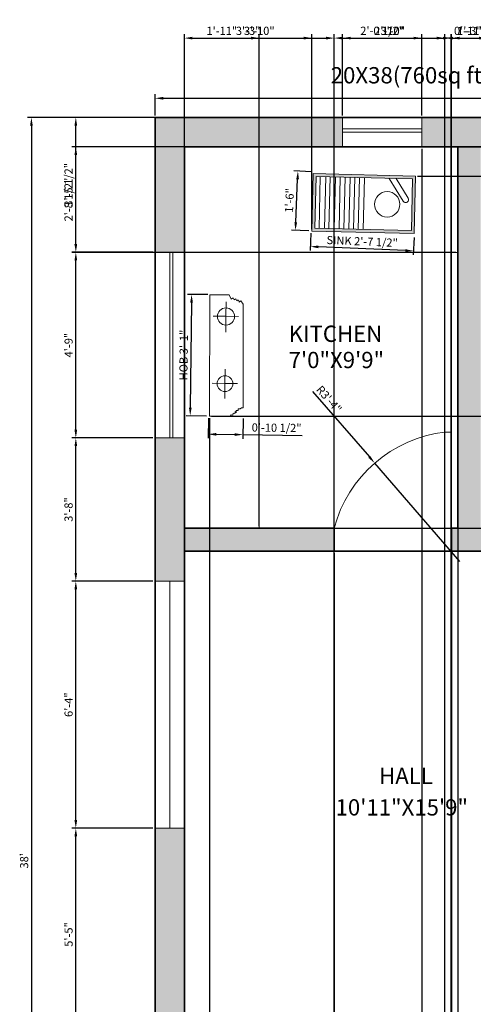
# Model space of a CAD drawing. Units: millimetres. Extents: x 2466 to 2817, y 2000 to 2512.
# Tile 3 of 4: x 2466 to 2605, y 2210 to 2512. Entities that reach past the tile are written whole.
import ezdxf

# ---------------------------------------------------------------- set-up
doc = ezdxf.new("R2010")
doc.units = ezdxf.units.MM
for name, color, linetype, lineweight in [('A-ANNO-DIMS', 2, 'Continuous', 13), ('A-ANNO-TEXT', 7, 'Continuous', 18), ('A-AREA-IDEN', 7, 'Continuous', 18), ('A-DOOR', 3, 'Continuous', 18), ('A-EQPM', 8, 'Continuous', 18), ('A-FLOR-FIXT', 9, 'Continuous', 18), ('A-GLAZ', 5, 'Continuous', 18), ('A-WALL', 7, 'Continuous', 35), ('A-WALL-PATT', 8, 'Continuous', 13)]:
    doc.layers.add(name, color=color, linetype=linetype, lineweight=lineweight)
doc.styles.get("Standard").update_dxf_attribs({"font": 'arial.ttf'})
doc.dimstyles.new('ISO-25', dxfattribs={"dimtxt": 2.5, "dimasz": 2.5, "dimexe": 1.25, "dimexo": 0.625, "dimtad": 1, "dimdec": 0, "dimlunit": 3, "dimtxsty": 'Standard', "dimcen": 2.5, "dimadec": 0, "dimazin": 0, "dimtfac": 1, "dimtdec": 0, "dimtmove": 0, "dimatfit": 3, "dimfxl": 1, "dimarcsym": 0})

# ---------------------------------------------------------------- blocks, each defined once
blk = doc.blocks.new('oven')
h = blk.add_hatch(color=256)
h.dxf.hatch_style = 1
h.paths.add_polyline_path([(0, 0), (-0.57, 31.4), (-18.19, 31.08), (-17.62, -0.32)])
h.paths.add_polyline_path([(-0.89, 0.86), (-16.76, 0.57), (-17.3, 30.22), (-1.42, 30.51)], flags=16)
h.paths.add_polyline_path([(-8.94, 4.45, -1), (-9.08, 12.23, -1)], flags=0)
for p, q in [((-1.42, 30.51), (-17.3, 30.22)), ((-1.4, 29.22), (-17.27, 28.94)), ((-1.37, 27.54), (-17.24, 27.26)), ((-1.35, 26.2), (-17.22, 25.91)), ((-1.32, 24.58), (-17.19, 24.29)), ((-1.29, 23.09), (-17.16, 22.8)), ((-1.26, 21.61), (-17.14, 21.33)), ((-1.24, 20.06), (-17.11, 19.77)), ((-1.21, 18.65), (-17.08, 18.36)), ((-1.19, 17.21), (-17.06, 16.92)), ((-1.16, 15.68), (-17.03, 15.4)), ((-1.02, 8.05), (-7.83, 3.46)), ((-8.14, 3.25), (-8.14, 3.25)), ((-0.98, 5.97), (-6.86, 2.02))]:
    blk.add_line(p, q)
for points in [[(-0.57, 31.4), (0, 0), (-17.62, -0.32), (-18.19, 31.08)], [(-1.42, 30.51), (-0.89, 0.86), (-16.76, 0.57), (-17.3, 30.22)]]:
    blk.add_lwpolyline(points, close=True)
blk.add_circle((-9.01, 8.34), 3.89)
blk.add_arc((-7.34, 2.74), 0.871, 123.9581, 303.9581)
blk = doc.blocks.new('gas stove')
for p, q in [((-59.95, 17.3), (-4.61, 17.86)), ((-4.61, 16.99), (-4.61, 17.86)), ((-4.03, 16.21), (-4.61, 16.99)), ((-4, 15.26), (-4.03, 16.21)), ((-0.18, 17.9), (-0.16, 17.9)), ((-53.37, 8.07), (-53.37, 14.75)), ((-53.37, 14.75), (-53.37, 1.35)), ((-17.48, 7.97), (-17.48, 14.65)), ((-17.48, 14.65), (-17.48, 1.25)), ((-3.18, 15.29), (-4, 15.26)), ((-3.15, 14.19), (-3.18, 15.29)), ((-1.96, 14.22), (-3.15, 14.19)), ((-2.6, 13.68), (-1.96, 14.22)), ((-1.52, 13.51), (-2.6, 13.68)), ((-1.66, 12.63), (-1.52, 13.51)), ((-0.57, 12.46), (-1.66, 12.63)), ((-0.73, 11.48), (-0.57, 12.46)), ((-0.11, 11.04), (-0.73, 11.48)), ((0, 0), (-0.11, 11.04)), ((0, 0), (-0.11, 11.04)), ((-64.71, -0.66), (-64.81, 9.74)), ((-64.71, -0.66), (-64.81, 9.74)), ((-53.37, 8.05), (-61.06, 8.07)), ((-53.37, 8.07), (-44.91, 8.07)), ((-53.37, 1.35), (-53.37, 8.05)), ((-17.48, 7.95), (-25.17, 7.97)), ((-17.48, 7.97), (-9.38, 7.97)), ((-17.48, 1.25), (-17.48, 7.95)), ((-64.71, -0.66), (0, 0))]:
    blk.add_line(p, q)
blk.add_lwpolyline([(-64.81, 9.74), (-62.59, 10.77), (-62.59, 10.77), (-63.19, 11.79), (-62.17, 12.38), (-62.65, 13.21), (-61.69, 13.77), (-62.14, 14.54), (-60.96, 15.22), (-61.23, 15.06), (-61.72, 15.9), (-59.95, 17.3)])
for centre, radius in [((-53.26, 8.13), 4.57), ((-17.38, 8.02), 4.19)]:
    blk.add_circle(centre, radius)
blk = doc.blocks.new('*D9')
at = {"layer": 'A-ANNO-DIMS', "color": 0, "lineweight": -2, "transparency": 16777216}
for p, q in [((2507.19, 2482.77), (2507.19, 2489.26)), ((2747.19, 2482.77), (2747.19, 2489.26)), ((2509.69, 2488.01), (2744.69, 2488.01))]:
    blk.add_line(p, q, dxfattribs=at)
at = {"layer": 'A-ANNO-DIMS', "color": 0, "transparency": 16777216}
for points in [[(2509.69, 2488.43), (2509.69, 2487.6), (2507.19, 2488.01)], [(2744.69, 2488.43), (2744.69, 2487.6), (2747.19, 2488.01)]]:
    blk.add_solid(points, dxfattribs=at)
at = {"layer": 'Defpoints', "color": 0, "transparency": 16777216}
for p in [(2747.19, 2488.01), (2507.19, 2482.15), (2747.19, 2482.15)]:
    blk.add_point(p, dxfattribs=at)
at = {"layer": 'A-ANNO-DIMS', "color": 0, "transparency": 16777216, "insert": (2627.19, 2489.92), "char_height": 2.5, "attachment_point": 5}
blk.add_mtext("20'", dxfattribs=at)
blk = doc.blocks.new('*D10')
at = {"layer": 'A-ANNO-DIMS', "color": 0, "lineweight": -2, "transparency": 16777216}
for p, q in [((2746.56, 2482.15), (2467.98, 2482.15)), ((2469.23, 2479.65), (2469.23, 2028.65)), ((2746.56, 2026.15), (2467.98, 2026.15))]:
    blk.add_line(p, q, dxfattribs=at)
at = {"layer": 'A-ANNO-DIMS', "color": 0, "transparency": 16777216}
for points in [[(2468.82, 2479.65), (2469.65, 2479.65), (2469.23, 2482.15)], [(2468.82, 2028.65), (2469.65, 2028.65), (2469.23, 2026.15)]]:
    blk.add_solid(points, dxfattribs=at)
at = {"layer": 'Defpoints', "color": 0, "transparency": 16777216}
for p in [(2747.19, 2482.15), (2469.23, 2026.15), (2747.19, 2026.15)]:
    blk.add_point(p, dxfattribs=at)
at = {"layer": 'A-ANNO-DIMS', "color": 0, "transparency": 16777216, "insert": (2467.33, 2254.15), "char_height": 2.5, "attachment_point": 5, "rotation": 90}
blk.add_mtext("38'", dxfattribs=at)
blk = doc.blocks.new('*D14')
at = {"layer": 'A-ANNO-DIMS', "color": 0, "lineweight": -2, "transparency": 16777216}
for p, q in [((2523.38, 2427.8), (2517.18, 2427.87)), ((2518.4, 2425.35), (2518.02, 2393.13)), ((2522.95, 2390.57), (2516.74, 2390.64))]:
    blk.add_line(p, q, dxfattribs=at)
at = {"layer": 'A-ANNO-DIMS', "color": 0, "transparency": 16777216}
for points in [[(2517.98, 2425.36), (2518.81, 2425.35), (2518.43, 2427.85)], [(2517.6, 2393.13), (2518.44, 2393.12), (2517.99, 2390.63)]]:
    blk.add_solid(points, dxfattribs=at)
at = {"layer": 'Defpoints', "color": 0, "transparency": 16777216}
for p in [(2524.01, 2427.79), (2517.99, 2390.63), (2523.58, 2390.56)]:
    blk.add_point(p, dxfattribs=at)
at = {"layer": 'A-ANNO-DIMS', "color": 0, "transparency": 16777216, "insert": (2516.29, 2409.26), "char_height": 2.5, "attachment_point": 5, "rotation": 89.3309}
blk.add_mtext('HOB 3\'-1"', dxfattribs=at)
blk = doc.blocks.new('*D15')
at = {"layer": 'A-ANNO-DIMS', "color": 0, "lineweight": -2, "transparency": 16777216}
for p, q in [((2523.57, 2389.94), (2523.5, 2383.73)), ((2534.23, 2389.81), (2534.16, 2383.6)), ((2526.01, 2384.95), (2531.67, 2384.88)), ((2534.17, 2384.85), (2552.33, 2384.64))]:
    blk.add_line(p, q, dxfattribs=at)
at = {"layer": 'A-ANNO-DIMS', "color": 0, "transparency": 16777216}
for points in [[(2526.01, 2385.37), (2526, 2384.53), (2523.51, 2384.98)], [(2531.68, 2385.3), (2531.67, 2384.47), (2534.17, 2384.85)]]:
    blk.add_solid(points, dxfattribs=at)
at = {"layer": 'Defpoints', "color": 0, "transparency": 16777216}
for p in [(2523.58, 2390.56), (2534.24, 2390.44), (2534.17, 2384.85)]:
    blk.add_point(p, dxfattribs=at)
at = {"layer": 'A-ANNO-DIMS', "color": 0, "transparency": 16777216, "insert": (2544.52, 2386.65), "char_height": 2.5, "attachment_point": 5, "rotation": 359.3309}
blk.add_mtext('0\'-10 1/2"', dxfattribs=at)
blk = doc.blocks.new('*D16')
at = {"layer": 'A-ANNO-DIMS', "color": 0, "lineweight": -2, "transparency": 16777216}
for p, q in [((2555.03, 2446.67), (2554.8, 2441.3)), ((2586.72, 2445.34), (2586.49, 2439.96)), ((2584.05, 2441.31), (2557.35, 2442.44))]:
    blk.add_line(p, q, dxfattribs=at)
at = {"layer": 'A-ANNO-DIMS', "color": 0, "transparency": 16777216}
for points in [[(2557.37, 2442.86), (2557.33, 2442.02), (2554.85, 2442.54)], [(2584.06, 2441.73), (2584.03, 2440.9), (2586.54, 2441.21)]]:
    blk.add_solid(points, dxfattribs=at)
at = {"layer": 'Defpoints', "color": 0, "transparency": 16777216}
for p in [(2555.05, 2447.3), (2586.74, 2445.96), (2554.85, 2442.54)]:
    blk.add_point(p, dxfattribs=at)
at = {"layer": 'A-ANNO-DIMS', "color": 0, "transparency": 16777216, "insert": (2570.78, 2443.79), "char_height": 2.5, "attachment_point": 5, "rotation": 357.5814}
blk.add_mtext('SINK 2\'-7 1/2"', dxfattribs=at)
blk = doc.blocks.new('*D17')
at = {"layer": 'A-ANNO-DIMS', "color": 0, "lineweight": -2, "transparency": 16777216}
for p, q in [((2555.2, 2465.5), (2549.82, 2465.72)), ((2550.41, 2450), (2550.96, 2463.17)), ((2554.43, 2447.32), (2549.05, 2447.55))]:
    blk.add_line(p, q, dxfattribs=at)
at = {"layer": 'A-ANNO-DIMS', "color": 0, "transparency": 16777216}
for points in [[(2550.55, 2463.19), (2551.38, 2463.15), (2551.07, 2465.67)], [(2549.99, 2450.01), (2550.82, 2449.98), (2550.3, 2447.5)]]:
    blk.add_solid(points, dxfattribs=at)
at = {"layer": 'Defpoints', "color": 0, "transparency": 16777216}
for p in [(2551.07, 2465.67), (2555.82, 2465.47), (2555.05, 2447.3)]:
    blk.add_point(p, dxfattribs=at)
at = {"layer": 'A-ANNO-DIMS', "color": 0, "transparency": 16777216, "insert": (2548.79, 2456.66), "char_height": 2.5, "attachment_point": 5, "rotation": 87.5814}
blk.add_mtext('1\'-6"', dxfattribs=at)
blk = doc.blocks.new('*D31')
at = {"layer": 'A-ANNO-DIMS', "color": 0, "lineweight": -2, "transparency": 16777216}
for p, q in [((2506.56, 2264.15), (2481.62, 2264.15)), ((2482.87, 2201.47), (2482.87, 2261.65)), ((2506.56, 2198.97), (2481.62, 2198.97))]:
    blk.add_line(p, q, dxfattribs=at)
at = {"layer": 'A-ANNO-DIMS', "color": 0, "transparency": 16777216}
for points in [[(2482.45, 2261.65), (2483.28, 2261.65), (2482.87, 2264.15)], [(2482.45, 2201.47), (2483.28, 2201.47), (2482.87, 2198.97)]]:
    blk.add_solid(points, dxfattribs=at)
at = {"layer": 'Defpoints', "color": 0, "transparency": 16777216}
for p in [(2482.87, 2264.15), (2507.19, 2264.15), (2507.19, 2198.97)]:
    blk.add_point(p, dxfattribs=at)
at = {"layer": 'A-ANNO-DIMS', "color": 0, "transparency": 16777216, "insert": (2480.97, 2231.56), "char_height": 2.5, "attachment_point": 5, "rotation": 90}
blk.add_mtext('5\'-5"', dxfattribs=at)
blk = doc.blocks.new('*D32')
at = {"layer": 'A-ANNO-DIMS', "color": 0, "lineweight": -2, "transparency": 16777216}
for p, q in [((2506.56, 2339.92), (2481.62, 2339.92)), ((2482.87, 2266.65), (2482.87, 2337.42)), ((2506.56, 2264.15), (2481.62, 2264.15))]:
    blk.add_line(p, q, dxfattribs=at)
at = {"layer": 'A-ANNO-DIMS', "color": 0, "transparency": 16777216}
for points in [[(2482.45, 2337.42), (2483.28, 2337.42), (2482.87, 2339.92)], [(2482.45, 2266.65), (2483.28, 2266.65), (2482.87, 2264.15)]]:
    blk.add_solid(points, dxfattribs=at)
at = {"layer": 'Defpoints', "color": 0, "transparency": 16777216}
for p in [(2482.87, 2339.92), (2507.19, 2339.92), (2507.19, 2264.15)]:
    blk.add_point(p, dxfattribs=at)
at = {"layer": 'A-ANNO-DIMS', "color": 0, "transparency": 16777216, "insert": (2480.97, 2302.03), "char_height": 2.5, "attachment_point": 5, "rotation": 90}
blk.add_mtext('6\'-4"', dxfattribs=at)
blk = doc.blocks.new('*D33')
at = {"layer": 'A-ANNO-DIMS', "color": 0, "lineweight": -2, "transparency": 16777216}
for p, q in [((2506.56, 2383.84), (2481.62, 2383.84)), ((2482.87, 2342.42), (2482.87, 2381.34)), ((2506.56, 2339.92), (2481.62, 2339.92))]:
    blk.add_line(p, q, dxfattribs=at)
at = {"layer": 'A-ANNO-DIMS', "color": 0, "transparency": 16777216}
for points in [[(2482.45, 2381.34), (2483.28, 2381.34), (2482.87, 2383.84)], [(2482.45, 2342.42), (2483.28, 2342.42), (2482.87, 2339.92)]]:
    blk.add_solid(points, dxfattribs=at)
at = {"layer": 'Defpoints', "color": 0, "transparency": 16777216}
for p in [(2482.87, 2383.84), (2507.19, 2383.84), (2507.19, 2339.92)]:
    blk.add_point(p, dxfattribs=at)
at = {"layer": 'A-ANNO-DIMS', "color": 0, "transparency": 16777216, "insert": (2480.96, 2361.88), "char_height": 2.5, "attachment_point": 5, "rotation": 90}
blk.add_mtext('3\'-8"', dxfattribs=at)
blk = doc.blocks.new('*D34')
at = {"layer": 'A-ANNO-DIMS', "color": 0, "lineweight": -2, "transparency": 16777216}
for p, q in [((2506.56, 2440.79), (2481.62, 2440.79)), ((2482.87, 2386.34), (2482.87, 2438.29)), ((2506.56, 2383.84), (2481.62, 2383.84))]:
    blk.add_line(p, q, dxfattribs=at)
at = {"layer": 'A-ANNO-DIMS', "color": 0, "transparency": 16777216}
for points in [[(2482.45, 2438.29), (2483.28, 2438.29), (2482.87, 2440.79)], [(2482.45, 2386.34), (2483.28, 2386.34), (2482.87, 2383.84)]]:
    blk.add_solid(points, dxfattribs=at)
at = {"layer": 'Defpoints', "color": 0, "transparency": 16777216}
for p in [(2482.87, 2440.79), (2507.19, 2440.79), (2507.19, 2383.84)]:
    blk.add_point(p, dxfattribs=at)
at = {"layer": 'A-ANNO-DIMS', "color": 0, "transparency": 16777216, "insert": (2480.97, 2412.31), "char_height": 2.5, "attachment_point": 5, "rotation": 90}
blk.add_mtext('4\'-9"', dxfattribs=at)
blk = doc.blocks.new('*D35')
at = {"layer": 'A-ANNO-DIMS', "color": 0, "lineweight": -2, "transparency": 16777216}
for p, q in [((2506.56, 2482.15), (2481.62, 2482.15)), ((2482.87, 2443.29), (2482.87, 2479.65)), ((2506.56, 2440.79), (2481.62, 2440.79))]:
    blk.add_line(p, q, dxfattribs=at)
at = {"layer": 'A-ANNO-DIMS', "color": 0, "transparency": 16777216}
for points in [[(2482.45, 2479.65), (2483.28, 2479.65), (2482.87, 2482.15)], [(2482.45, 2443.29), (2483.28, 2443.29), (2482.87, 2440.79)]]:
    blk.add_solid(points, dxfattribs=at)
at = {"layer": 'Defpoints', "color": 0, "transparency": 16777216}
for p in [(2482.87, 2482.15), (2507.19, 2482.15), (2507.19, 2440.79)]:
    blk.add_point(p, dxfattribs=at)
at = {"layer": 'A-ANNO-DIMS', "color": 0, "transparency": 16777216, "insert": (2480.95, 2461.47), "char_height": 2.5, "attachment_point": 5, "rotation": 90}
blk.add_mtext('3\'-5 1/2"', dxfattribs=at)
blk = doc.blocks.new('*D40')
at = {"layer": 'A-ANNO-DIMS', "color": 0, "lineweight": -2, "transparency": 16777216}
for p, q in [((2589.08, 2472.52), (2589.08, 2000.58)), ((2600.19, 2472.52), (2600.19, 2000.58)), ((2591.58, 2001.83), (2597.69, 2001.83))]:
    blk.add_line(p, q, dxfattribs=at)
at = {"layer": 'A-ANNO-DIMS', "color": 0, "transparency": 16777216}
for points in [[(2591.58, 2002.24), (2591.58, 2001.41), (2589.08, 2001.83)], [(2597.69, 2002.24), (2597.69, 2001.41), (2600.19, 2001.83)]]:
    blk.add_solid(points, dxfattribs=at)
at = {"layer": 'Defpoints', "color": 0, "transparency": 16777216}
for p in [(2589.08, 2473.15), (2600.19, 2473.15), (2600.19, 2001.83)]:
    blk.add_point(p, dxfattribs=at)
at = {"layer": 'A-ANNO-DIMS', "color": 0, "transparency": 16777216, "insert": (2594.63, 2003.73), "char_height": 2.5, "attachment_point": 5}
blk.add_mtext('0\'-11"', dxfattribs=at)
blk = doc.blocks.new('*D41')
at = {"layer": 'A-ANNO-DIMS', "color": 0, "lineweight": -2, "transparency": 16777216}
for p, q in [((2564.77, 2482.77), (2564.77, 2507.72)), ((2567.27, 2506.47), (2586.58, 2506.47)), ((2589.08, 2482.77), (2589.08, 2507.72))]:
    blk.add_line(p, q, dxfattribs=at)
at = {"layer": 'A-ANNO-DIMS', "color": 0, "transparency": 16777216}
for points in [[(2567.27, 2506.88), (2567.27, 2506.05), (2564.77, 2506.47)], [(2586.58, 2506.88), (2586.58, 2506.05), (2589.08, 2506.47)]]:
    blk.add_solid(points, dxfattribs=at)
at = {"layer": 'Defpoints', "color": 0, "transparency": 16777216}
for p in [(2589.08, 2506.47), (2564.77, 2482.15), (2589.08, 2482.15)]:
    blk.add_point(p, dxfattribs=at)
at = {"layer": 'A-ANNO-DIMS', "color": 0, "transparency": 16777216, "insert": (2576.93, 2508.39), "char_height": 2.5, "attachment_point": 5}
blk.add_mtext('2\'-0 1/2"', dxfattribs=at)
blk = doc.blocks.new('*D44')
at = {"layer": 'A-ANNO-DIMS', "color": 0, "lineweight": -2, "transparency": 16777216}
for p, q in [((2516.19, 2055.77), (2516.19, 2507.72)), ((2518.69, 2506.47), (2559.74, 2506.47)), ((2562.24, 2055.77), (2562.24, 2507.72))]:
    blk.add_line(p, q, dxfattribs=at)
at = {"layer": 'A-ANNO-DIMS', "color": 0, "transparency": 16777216}
for points in [[(2518.69, 2506.88), (2518.69, 2506.05), (2516.19, 2506.47)], [(2559.74, 2506.88), (2559.74, 2506.05), (2562.24, 2506.47)]]:
    blk.add_solid(points, dxfattribs=at)
at = {"layer": 'Defpoints', "color": 0, "transparency": 16777216}
for p in [(2562.24, 2506.47), (2516.19, 2055.15), (2562.24, 2055.15)]:
    blk.add_point(p, dxfattribs=at)
at = {"layer": 'A-ANNO-DIMS', "color": 0, "transparency": 16777216, "insert": (2539.21, 2508.37), "char_height": 2.5, "attachment_point": 5}
blk.add_mtext('3\'-10"', dxfattribs=at)
blk = doc.blocks.new('*D47')
at = {"layer": 'A-ANNO-DIMS', "color": 0, "lineweight": -2, "transparency": 16777216}
for p, q in [((2516.19, 2348.52), (2516.19, 2000.58)), ((2562.19, 2348.52), (2562.19, 2000.58)), ((2518.69, 2001.83), (2559.69, 2001.83))]:
    blk.add_line(p, q, dxfattribs=at)
at = {"layer": 'A-ANNO-DIMS', "color": 0, "transparency": 16777216}
for points in [[(2518.69, 2002.24), (2518.69, 2001.41), (2516.19, 2001.83)], [(2559.69, 2002.24), (2559.69, 2001.41), (2562.19, 2001.83)]]:
    blk.add_solid(points, dxfattribs=at)
at = {"layer": 'Defpoints', "color": 0, "transparency": 16777216}
for p in [(2516.19, 2349.15), (2562.19, 2349.15), (2562.19, 2001.83)]:
    blk.add_point(p, dxfattribs=at)
at = {"layer": 'A-ANNO-DIMS', "color": 0, "transparency": 16777216, "insert": (2539.19, 2003.73), "char_height": 2.5, "attachment_point": 5}
blk.add_mtext('3\'-10"', dxfattribs=at)
blk = doc.blocks.new('*D48')
at = {"layer": 'A-ANNO-DIMS', "color": 0, "lineweight": -2, "transparency": 16777216}
for p, q in [((2562.19, 2348.52), (2562.19, 2000.58)), ((2598.19, 2348.52), (2598.19, 2000.58)), ((2564.69, 2001.83), (2595.69, 2001.83))]:
    blk.add_line(p, q, dxfattribs=at)
at = {"layer": 'A-ANNO-DIMS', "color": 0, "transparency": 16777216}
for points in [[(2564.69, 2002.24), (2564.69, 2001.41), (2562.19, 2001.83)], [(2595.69, 2002.24), (2595.69, 2001.41), (2598.19, 2001.83)]]:
    blk.add_solid(points, dxfattribs=at)
at = {"layer": 'Defpoints', "color": 0, "transparency": 16777216}
for p in [(2562.19, 2349.15), (2598.19, 2349.15), (2598.19, 2001.83)]:
    blk.add_point(p, dxfattribs=at)
at = {"layer": 'A-ANNO-DIMS', "color": 0, "transparency": 16777216, "insert": (2580.19, 2003.73), "char_height": 2.5, "attachment_point": 5}
blk.add_mtext('3\'-0"', dxfattribs=at)
blk = doc.blocks.new('*D49')
at = {"layer": 'A-ANNO-DIMS', "color": 0, "lineweight": -2, "transparency": 16777216}
for p, q in [((2598.19, 2356.77), (2598.19, 2507.72)), ((2600.69, 2506.47), (2606.69, 2506.47)), ((2609.19, 2356.77), (2609.19, 2507.72))]:
    blk.add_line(p, q, dxfattribs=at)
at = {"layer": 'A-ANNO-DIMS', "color": 0, "transparency": 16777216}
for points in [[(2600.69, 2506.88), (2600.69, 2506.05), (2598.19, 2506.47)], [(2606.69, 2506.88), (2606.69, 2506.05), (2609.19, 2506.47)]]:
    blk.add_solid(points, dxfattribs=at)
at = {"layer": 'Defpoints', "color": 0, "transparency": 16777216}
for p in [(2609.19, 2506.47), (2598.19, 2356.15), (2609.19, 2356.15)]:
    blk.add_point(p, dxfattribs=at)
at = {"layer": 'A-ANNO-DIMS', "color": 0, "transparency": 16777216, "insert": (2603.69, 2508.37), "char_height": 2.5, "attachment_point": 5}
blk.add_mtext('0\'-11"', dxfattribs=at)
blk = doc.blocks.new('*D51')
at = {"layer": 'A-ANNO-DIMS', "color": 0, "lineweight": -2, "transparency": 16777216}
for p, q in [((2516.19, 2155.77), (2516.19, 2507.72)), ((2518.69, 2506.47), (2559.69, 2506.47)), ((2562.19, 2155.77), (2562.19, 2507.72))]:
    blk.add_line(p, q, dxfattribs=at)
at = {"layer": 'A-ANNO-DIMS', "color": 0, "transparency": 16777216}
for points in [[(2518.69, 2506.88), (2518.69, 2506.05), (2516.19, 2506.47)], [(2559.69, 2506.88), (2559.69, 2506.05), (2562.19, 2506.47)]]:
    blk.add_solid(points, dxfattribs=at)
at = {"layer": 'Defpoints', "color": 0, "transparency": 16777216}
for p in [(2562.19, 2506.47), (2516.19, 2155.15), (2562.19, 2155.15)]:
    blk.add_point(p, dxfattribs=at)
at = {"layer": 'A-ANNO-DIMS', "color": 0, "transparency": 16777216, "insert": (2539.19, 2508.37), "char_height": 2.5, "attachment_point": 5}
blk.add_mtext('3\'-10"', dxfattribs=at)
blk = doc.blocks.new('*D52')
at = {"layer": 'A-ANNO-DIMS', "color": 0, "lineweight": -2, "transparency": 16777216}
for p, q in [((2562.19, 2155.77), (2562.19, 2507.72)), ((2564.69, 2506.47), (2593.69, 2506.47)), ((2596.19, 2155.77), (2596.19, 2507.72))]:
    blk.add_line(p, q, dxfattribs=at)
at = {"layer": 'A-ANNO-DIMS', "color": 0, "transparency": 16777216}
for points in [[(2564.69, 2506.88), (2564.69, 2506.05), (2562.19, 2506.47)], [(2593.69, 2506.88), (2593.69, 2506.05), (2596.19, 2506.47)]]:
    blk.add_solid(points, dxfattribs=at)
at = {"layer": 'Defpoints', "color": 0, "transparency": 16777216}
for p in [(2596.19, 2506.47), (2562.19, 2155.15), (2596.19, 2155.15)]:
    blk.add_point(p, dxfattribs=at)
at = {"layer": 'A-ANNO-DIMS', "color": 0, "transparency": 16777216, "insert": (2579.19, 2508.37), "char_height": 2.5, "attachment_point": 5}
blk.add_mtext('2\'-10"', dxfattribs=at)
blk = doc.blocks.new('*D53')
at = {"layer": 'A-ANNO-DIMS', "color": 0, "lineweight": -2, "transparency": 16777216}
for p, q in [((2596.19, 2155.77), (2596.19, 2507.72)), ((2598.69, 2506.47), (2608.69, 2506.47)), ((2611.19, 2155.77), (2611.19, 2507.72))]:
    blk.add_line(p, q, dxfattribs=at)
at = {"layer": 'A-ANNO-DIMS', "color": 0, "transparency": 16777216}
for points in [[(2598.69, 2506.88), (2598.69, 2506.05), (2596.19, 2506.47)], [(2608.69, 2506.88), (2608.69, 2506.05), (2611.19, 2506.47)]]:
    blk.add_solid(points, dxfattribs=at)
at = {"layer": 'Defpoints', "color": 0, "transparency": 16777216}
for p in [(2611.19, 2506.47), (2596.19, 2155.15), (2611.19, 2155.15)]:
    blk.add_point(p, dxfattribs=at)
at = {"layer": 'A-ANNO-DIMS', "color": 0, "transparency": 16777216, "insert": (2603.69, 2508.37), "char_height": 2.5, "attachment_point": 5}
blk.add_mtext('1\'-3"', dxfattribs=at)
blk = doc.blocks.new('*D64')
at = {"layer": 'A-ANNO-DIMS', "color": 0, "lineweight": -2, "transparency": 16777216}
for p, q in [((2562.24, 2055.77), (2562.24, 2507.72)), ((2564.74, 2506.47), (2595.62, 2506.47)), ((2598.12, 2055.77), (2598.12, 2507.72))]:
    blk.add_line(p, q, dxfattribs=at)
at = {"layer": 'A-ANNO-DIMS', "color": 0, "transparency": 16777216}
for points in [[(2564.74, 2506.88), (2564.74, 2506.05), (2562.24, 2506.47)], [(2595.62, 2506.88), (2595.62, 2506.05), (2598.12, 2506.47)]]:
    blk.add_solid(points, dxfattribs=at)
at = {"layer": 'Defpoints', "color": 0, "transparency": 16777216}
for p in [(2598.12, 2506.47), (2562.24, 2055.15), (2598.12, 2055.15)]:
    blk.add_point(p, dxfattribs=at)
at = {"layer": 'A-ANNO-DIMS', "color": 0, "transparency": 16777216, "insert": (2580.18, 2508.37), "char_height": 2.5, "attachment_point": 5}
blk.add_mtext('3\'-0"', dxfattribs=at)
blk = doc.blocks.new('*D65')
at = {"layer": 'A-ANNO-DIMS', "color": 0, "lineweight": -2, "transparency": 16777216}
for p, q in [((2516.19, 2356.77), (2516.19, 2507.72)), ((2518.69, 2506.47), (2536.69, 2506.47)), ((2539.19, 2356.77), (2539.19, 2507.72))]:
    blk.add_line(p, q, dxfattribs=at)
at = {"layer": 'A-ANNO-DIMS', "color": 0, "transparency": 16777216}
for points in [[(2518.69, 2506.88), (2518.69, 2506.05), (2516.19, 2506.47)], [(2536.69, 2506.88), (2536.69, 2506.05), (2539.19, 2506.47)]]:
    blk.add_solid(points, dxfattribs=at)
at = {"layer": 'Defpoints', "color": 0, "transparency": 16777216}
for p in [(2539.19, 2506.47), (2516.19, 2356.15), (2539.19, 2356.15)]:
    blk.add_point(p, dxfattribs=at)
at = {"layer": 'A-ANNO-DIMS', "color": 0, "transparency": 16777216, "insert": (2527.69, 2508.35), "char_height": 2.5, "attachment_point": 5}
blk.add_mtext('1\'-11"', dxfattribs=at)
blk = doc.blocks.new('*D66')
at = {"layer": 'A-ANNO-DIMS', "color": 0, "lineweight": -2, "transparency": 16777216}
for p, q in [((2599.56, 2473.15), (2481.62, 2473.15)), ((2482.87, 2443.24), (2482.87, 2470.65)), ((2599.56, 2440.74), (2481.62, 2440.74))]:
    blk.add_line(p, q, dxfattribs=at)
at = {"layer": 'A-ANNO-DIMS', "color": 0, "transparency": 16777216}
for points in [[(2482.45, 2470.65), (2483.28, 2470.65), (2482.87, 2473.15)], [(2482.45, 2443.24), (2483.28, 2443.24), (2482.87, 2440.74)]]:
    blk.add_solid(points, dxfattribs=at)
at = {"layer": 'Defpoints', "color": 0, "transparency": 16777216}
for p in [(2482.87, 2473.15), (2600.19, 2473.15), (2600.19, 2440.74)]:
    blk.add_point(p, dxfattribs=at)
at = {"layer": 'A-ANNO-DIMS', "color": 0, "transparency": 16777216, "insert": (2480.95, 2456.95), "char_height": 2.5, "attachment_point": 5, "rotation": 90}
blk.add_mtext('2\'-8 1/2"', dxfattribs=at)
blk = doc.blocks.new('*D69')
at = {"layer": 'A-ANNO-DIMS', "color": 0, "lineweight": -2, "transparency": 16777216}
for p, q in [((2516.19, 2441.42), (2516.19, 2507.72)), ((2518.69, 2506.47), (2552.87, 2506.47)), ((2555.37, 2447.91), (2555.37, 2507.72))]:
    blk.add_line(p, q, dxfattribs=at)
at = {"layer": 'A-ANNO-DIMS', "color": 0, "transparency": 16777216}
for points in [[(2518.69, 2506.88), (2518.69, 2506.05), (2516.19, 2506.47)], [(2552.87, 2506.88), (2552.87, 2506.05), (2555.37, 2506.47)]]:
    blk.add_solid(points, dxfattribs=at)
at = {"layer": 'Defpoints', "color": 0, "transparency": 16777216}
for p in [(2555.37, 2506.47), (2555.37, 2447.28), (2516.19, 2440.79)]:
    blk.add_point(p, dxfattribs=at)
at = {"layer": 'A-ANNO-DIMS', "color": 0, "transparency": 16777216, "insert": (2535.78, 2508.37), "char_height": 2.5, "attachment_point": 5}
blk.add_mtext('3\'-3"', dxfattribs=at)
blk = doc.blocks.new('*D70')
at = {"layer": 'A-ANNO-DIMS', "color": 0, "lineweight": -2, "transparency": 16777216}
for p, q in [((2524.58, 2390.56), (2816.76, 2390.56)), ((2815.51, 2358.65), (2815.51, 2388.06)), ((2516.81, 2356.15), (2816.76, 2356.15))]:
    blk.add_line(p, q, dxfattribs=at)
at = {"layer": 'A-ANNO-DIMS', "color": 0, "transparency": 16777216}
for points in [[(2815.09, 2388.06), (2815.92, 2388.06), (2815.51, 2390.56)], [(2815.09, 2358.65), (2815.92, 2358.65), (2815.51, 2356.15)]]:
    blk.add_solid(points, dxfattribs=at)
at = {"layer": 'Defpoints', "color": 0, "transparency": 16777216}
for p in [(2523.95, 2390.56), (2815.51, 2390.56), (2516.19, 2356.15)]:
    blk.add_point(p, dxfattribs=at)
at = {"layer": 'A-ANNO-DIMS', "color": 0, "transparency": 16777216, "insert": (2813.59, 2373.35), "char_height": 2.5, "attachment_point": 5, "rotation": 90}
blk.add_mtext('2\'-10 1/2"', dxfattribs=at)
blk = doc.blocks.new('*D71')
at = {"layer": 'A-ANNO-DIMS', "color": 0, "lineweight": -2, "transparency": 16777216}
for p, q in [((2523.95, 2389.93), (2523.95, 2000.58)), ((2516.19, 2383.21), (2516.19, 2000.58)), ((2518.69, 2001.83), (2521.45, 2001.83)), ((2523.95, 2001.83), (2534.35, 2001.83))]:
    blk.add_line(p, q, dxfattribs=at)
at = {"layer": 'A-ANNO-DIMS', "color": 0, "transparency": 16777216}
for points in [[(2518.69, 2002.24), (2518.69, 2001.41), (2516.19, 2001.83)], [(2521.45, 2002.24), (2521.45, 2001.41), (2523.95, 2001.83)]]:
    blk.add_solid(points, dxfattribs=at)
at = {"layer": 'Defpoints', "color": 0, "transparency": 16777216}
for p in [(2523.95, 2390.56), (2516.19, 2383.84), (2523.95, 2001.83)]:
    blk.add_point(p, dxfattribs=at)
at = {"layer": 'A-ANNO-DIMS', "color": 0, "transparency": 16777216, "insert": (2530.4, 2003.73), "char_height": 2.5, "attachment_point": 5}
blk.add_mtext('0\'-8"', dxfattribs=at)
blk = doc.blocks.new('*D72')
at = {"layer": 'A-ANNO-DIMS', "color": 0, "lineweight": -2, "transparency": 16777216}
for p, q in [((2589.71, 2473.15), (2816.76, 2473.15)), ((2815.51, 2470.65), (2815.51, 2466.64)), ((2587.82, 2464.14), (2816.76, 2464.14))]:
    blk.add_line(p, q, dxfattribs=at)
at = {"layer": 'A-ANNO-DIMS', "color": 0, "transparency": 16777216}
for points in [[(2815.09, 2470.65), (2815.92, 2470.65), (2815.51, 2473.15)], [(2815.09, 2466.64), (2815.92, 2466.64), (2815.51, 2464.14)]]:
    blk.add_solid(points, dxfattribs=at)
at = {"layer": 'Defpoints', "color": 0, "transparency": 16777216}
for p in [(2589.08, 2473.15), (2587.19, 2464.14), (2815.51, 2464.14)]:
    blk.add_point(p, dxfattribs=at)
at = {"layer": 'A-ANNO-DIMS', "color": 0, "transparency": 16777216, "insert": (2813.61, 2468.65), "char_height": 2.5, "attachment_point": 5, "rotation": 90}
blk.add_mtext('0\'-9"', dxfattribs=at)
blk = doc.blocks.new('*D73')
at = {"layer": 'A-ANNO-DIMS', "color": 0, "lineweight": -2, "transparency": 16777216}
for p, q in [((2555.57, 2398.13), (2573, 2378.02)), ((2600.82, 2345.94), (2574.64, 2376.13))]:
    blk.add_line(p, q, dxfattribs=at)
at = {"layer": 'A-ANNO-DIMS', "color": 0, "transparency": 16777216}
blk.add_solid([(2573.32, 2378.29), (2572.69, 2377.75), (2574.64, 2376.13)], dxfattribs=at)
at = {"layer": 'Defpoints', "color": 0, "transparency": 16777216}
for p in [(2574.64, 2376.13), (2600.82, 2345.94)]:
    blk.add_point(p, dxfattribs=at)
at = {"layer": 'A-ANNO-DIMS', "color": 0, "transparency": 16777216, "insert": (2560.37, 2395.49), "char_height": 2.5, "attachment_point": 5, "rotation": 310.9284}
blk.add_mtext('R3\'-4"', dxfattribs=at)

msp = doc.modelspace()

# ---------------------------------------------------------------- hatches: boundary and pattern name
at = {"layer": 'A-WALL-PATT'}
h = msp.add_hatch(color=256, dxfattribs=at)
h.dxf.hatch_style = 1
h.paths.add_polyline_path([(2747.19, 2482.15), (2589.08, 2482.15), (2589.08, 2473.15), (2639.87, 2473.15), (2639.87, 2473.28), (2705.56, 2473.28), (2738.19, 2473.15), (2738.19, 2450.08), (2747.19, 2450.08)])
h.paths.add_polyline_path([(2564.77, 2482.15), (2507.19, 2482.15), (2507.19, 2440.79), (2516.19, 2440.79), (2516.19, 2473.15), (2564.77, 2473.15)])
h.paths.add_polyline_path([(2516.19, 2383.84), (2507.19, 2383.84), (2507.19, 2339.92), (2516.19, 2339.92)])
h.paths.add_polyline_path([(2607.19, 2473.15), (2600.19, 2473.15), (2600.19, 2356.15), (2607.19, 2356.15)])
h.paths.add_polyline_path([(2747.19, 2391.65), (2738.19, 2391.65), (2738.19, 2334.57), (2747.19, 2334.57)])
h = msp.add_hatch(color=256, dxfattribs=at)
h.dxf.hatch_style = 1
h.paths.add_polyline_path([(2562.19, 2356.15), (2516.19, 2356.15), (2516.19, 2349.15), (2562.19, 2349.15)])
h.paths.add_polyline_path([(2738.19, 2356.15), (2692.19, 2356.15), (2692.19, 2349.15), (2738.19, 2349.15)], flags=17)
h.paths.add_polyline_path([(2656.19, 2356.15), (2645.19, 2356.15), (2645.19, 2349.15), (2647.19, 2349.15), (2647.19, 2294.15), (2738.19, 2294.15), (2747.19, 2294.15), (2747.19, 2301.15), (2738.19, 2301.15), (2654.19, 2301.15), (2654.19, 2349.15), (2656.19, 2349.15)])
h = msp.add_hatch(color=256, dxfattribs=at)
h.dxf.hatch_style = 1
h.paths.add_polyline_path([(2609.19, 2356.15), (2607.19, 2356.15), (2598.19, 2356.15), (2598.19, 2349.15), (2609.19, 2349.15)])
h = msp.add_hatch(color=256, dxfattribs=at)
h.dxf.hatch_style = 1
h.paths.add_polyline_path([(2516.19, 2264.15), (2507.19, 2264.15), (2507.19, 2198.97), (2516.19, 2198.97)])

# ---------------------------------------------------------------- linework, layer by layer
at = {"layer": 'A-DOOR'}
for p, q in [((2598.19, 2385.63), (2596.19, 2385.63)), ((2596.19, 2385.63), (2596.19, 2349.15)), ((2598.19, 2356.15), (2598.19, 2385.63))]:
    msp.add_line(p, q, dxfattribs=at)
msp.add_arc((2600.82, 2345.94), 39.96, 96.6585, 165.1984, dxfattribs=at)
at = {"layer": 'A-FLOR-FIXT'}
for p, q in [((2539.19, 2356.15), (2539.19, 2440.74)), ((2539.19, 2440.74), (2600.19, 2440.74)), ((2539.19, 2356.15), (2539.19, 2356.15))]:
    msp.add_line(p, q, dxfattribs=at)
at = {"layer": 'A-GLAZ'}
for p, q in [((2589.08, 2482.15), (2564.77, 2482.15)), ((2564.77, 2482.15), (2564.77, 2473.15)), ((2589.08, 2482.15), (2589.08, 2473.15)), ((2589.08, 2478.65), (2564.77, 2478.65)), ((2589.08, 2477.65), (2564.77, 2477.65)), ((2564.77, 2473.15), (2589.08, 2473.15)), ((2516.19, 2440.79), (2507.19, 2440.79)), ((2507.19, 2440.79), (2507.19, 2383.84)), ((2511.69, 2440.79), (2511.69, 2383.84)), ((2512.69, 2440.79), (2512.69, 2383.84)), ((2516.19, 2383.84), (2516.19, 2440.79)), ((2507.19, 2383.84), (2516.19, 2383.84)), ((2516.19, 2339.92), (2507.19, 2339.92)), ((2507.19, 2339.92), (2507.19, 2265.15)), ((2511.69, 2339.92), (2511.69, 2264.65)), ((2516.19, 2264.15), (2516.19, 2339.92)), ((2507.19, 2265.15), (2507.19, 2264.15)), ((2516.19, 2264.15), (2507.19, 2264.15)), ((2511.69, 2264.65), (2511.69, 2264.15))]:
    msp.add_line(p, q, dxfattribs=at)
at = {"layer": 'A-WALL'}
for p, q in [((2507.19, 2482.15), (2747.19, 2482.15)), ((2507.19, 2048.15), (2507.19, 2482.15)), ((2516.19, 2473.15), (2738.19, 2473.15)), ((2516.19, 2055.15), (2516.19, 2473.15)), ((2600.19, 2356.15), (2600.19, 2473.15)), ((2516.19, 2356.15), (2562.19, 2356.15)), ((2562.19, 2356.15), (2562.19, 2349.15)), ((2600.19, 2356.15), (2598.19, 2356.15)), ((2598.19, 2356.15), (2598.19, 2349.15)), ((2598.19, 2356.15), (2600.19, 2356.15)), ((2516.19, 2349.15), (2609.19, 2349.15))]:
    msp.add_line(p, q, dxfattribs=at)

# ---------------------------------------------------------------- block references
at = {"layer": 'A-EQPM', "xscale": 0.5744135972665616, "yscale": 0.5744135972665616, "zscale": 0.5744135972665616, "rotation": 269.3308967307994}
msp.add_blockref('gas stove', (2523.95, 2390.56), dxfattribs=at)
at = {"layer": 'A-FLOR-FIXT', "rotation": 87.58144511676959}
msp.add_blockref('oven', (2587.19, 2464.14), dxfattribs=at)

# ---------------------------------------------------------------- texts
at = {"layer": 'A-ANNO-TEXT'}
msp.add_text('20X38(760sq ft)House Plan -North Face', height=5, dxfattribs=at).set_placement((2561.14, 2492.57))
at = {"layer": 'A-AREA-IDEN'}
for s, p in [('KITCHEN', (2548.22, 2413.29)), ('7\'0"X9\'9"', (2548.22, 2405.25)), ('HALL', (2575.98, 2277.69)), ('10\'11"X15\'9"', (2562.62, 2268.05))]:
    msp.add_text(s, height=5, dxfattribs=at).set_placement(p)

# ---------------------------------------------------------------- dimensions: what is measured, and where the dimension line sits
at = {"layer": 'A-ANNO-DIMS'}
for base, p1, p2, override, picture, middle in [((2562.2416, 2506.4679), (2516.1868, 2055.1479), (2562.2416, 2055.1479), {"dimdec": 1, "dimlfac": 1, "dimrnd": 0, "dimzin": 1, "dimdsep": 46, "dimlunit": 4, "dimfrac": 2}, '*D44', (2539.2142, 2508.3702)), ((2562.19, 2506.47), (2516.19, 2155.15), (2562.19, 2155.15), {"dimdec": 1, "dimlfac": 1, "dimrnd": 0, "dimzin": 1, "dimdsep": 46, "dimlunit": 4, "dimfrac": 2}, '*D51', (2539.19, 2508.37)), ((2555.37, 2506.47), (2516.19, 2440.79), (2555.37, 2447.28), {"dimdec": 1, "dimlfac": 1, "dimrnd": 0, "dimzin": 1, "dimdsep": 46, "dimlunit": 4, "dimfrac": 2}, '*D69', (2535.78, 2508.37)), ((2539.19, 2506.47), (2516.19, 2356.15), (2539.19, 2356.15), {"dimdec": 1, "dimlfac": 1, "dimrnd": 0, "dimzin": 1, "dimdsep": 46, "dimlunit": 4, "dimfrac": 2}, '*D65', (2527.69, 2508.35)), ((2596.19, 2506.47), (2562.19, 2155.15), (2596.19, 2155.15), {"dimdec": 1, "dimlfac": 1, "dimrnd": 0, "dimzin": 1, "dimdsep": 46, "dimlunit": 4, "dimfrac": 2}, '*D52', (2579.19, 2508.37)), ((2598.12, 2506.47), (2562.24, 2055.15), (2598.12, 2055.15), {"dimdec": 1, "dimlfac": 1, "dimrnd": 0, "dimzin": 1, "dimdsep": 46, "dimlunit": 4, "dimfrac": 2}, '*D64', (2580.18, 2508.37)), ((2589.08, 2506.47), (2564.77, 2482.15), (2589.08, 2482.15), {"dimdec": 1, "dimlfac": 1, "dimrnd": 0, "dimzin": 1, "dimdsep": 46, "dimlunit": 4, "dimfrac": 2}, '*D41', (2576.93, 2508.39)), ((2611.19, 2506.47), (2596.19, 2155.15), (2611.19, 2155.15), {"dimdec": 1, "dimlfac": 1, "dimrnd": 0, "dimzin": 1, "dimdsep": 46, "dimlunit": 4, "dimfrac": 2}, '*D53', (2603.69, 2508.37)), ((2609.19, 2506.47), (2598.19, 2356.15), (2609.19, 2356.15), {"dimdec": 1, "dimlfac": 1, "dimrnd": 0, "dimzin": 1, "dimdsep": 46, "dimlunit": 4, "dimfrac": 2}, '*D49', (2603.69, 2508.37)), ((2747.19, 2488.01), (2507.19, 2482.15), (2747.19, 2482.15), {"dimclrd": 0, "dimclre": 0, "dimclrt": 0}, '*D9', (2627.19, 2489.92)), ((2600.19, 2001.83), (2589.08, 2473.15), (2600.19, 2473.15), {"dimdec": 1, "dimlfac": 1, "dimrnd": 0, "dimzin": 1, "dimdsep": 46, "dimlunit": 4, "dimfrac": 2}, '*D40', (2594.63, 2003.73)), ((2523.95, 2001.83), (2516.19, 2383.84), (2523.95, 2390.56), {"dimdec": 1, "dimlfac": 1, "dimrnd": 0, "dimzin": 1, "dimdsep": 46, "dimlunit": 4, "dimfrac": 2}, '*D71', (2530.4, 2003.73)), ((2562.19, 2001.83), (2516.19, 2349.15), (2562.19, 2349.15), {"dimdec": 1, "dimlfac": 1, "dimrnd": 0, "dimzin": 1, "dimdsep": 46, "dimlunit": 4, "dimfrac": 2}, '*D47', (2539.19, 2003.73)), ((2598.19, 2001.83), (2562.19, 2349.15), (2598.19, 2349.15), {"dimdec": 1, "dimlfac": 1, "dimrnd": 0, "dimzin": 1, "dimdsep": 46, "dimlunit": 4, "dimfrac": 2}, '*D48', (2580.19, 2003.73))]:
    dim = msp.add_linear_dim(base=base, p1=p1, p2=p2, dimstyle='ISO-25', override=override, dxfattribs=at)
    dim.commit()
    dim.dimension.update_dxf_attribs({"geometry": picture, "text_midpoint": middle})
for base, p1, p2, angle, override, picture, middle in [((2469.23, 2026.15), (2747.19, 2482.15), (2747.19, 2026.15), 90, {"dimclrd": 0, "dimclre": 0, "dimclrt": 0}, '*D10', (2467.33, 2254.15)), ((2482.87, 2482.15), (2507.19, 2440.79), (2507.19, 2482.15), 90, {"dimdec": 1, "dimlfac": 1, "dimrnd": 0, "dimzin": 1, "dimdsep": 46, "dimlunit": 4, "dimfrac": 2}, '*D35', (2480.95, 2461.47)), ((2482.87, 2473.15), (2600.19, 2440.74), (2600.19, 2473.15), 90, {"dimdec": 1, "dimlfac": 1, "dimrnd": 0, "dimzin": 1, "dimdsep": 46, "dimlunit": 4, "dimfrac": 2}, '*D66', (2480.95, 2456.95)), ((2815.51, 2464.14), (2589.08, 2473.15), (2587.19, 2464.14), 90, {"dimdec": 1, "dimlfac": 1, "dimrnd": 0, "dimzin": 1, "dimdsep": 46, "dimlunit": 4, "dimfrac": 2}, '*D72', (2813.61, 2468.65)), ((2551.07, 2465.67), (2555.05, 2447.3), (2555.82, 2465.47), 87.5814, {"dimdec": 1, "dimlfac": 1, "dimrnd": 0, "dimzin": 1, "dimdsep": 46, "dimlunit": 4, "dimfrac": 2}, '*D17', (2548.79, 2456.66)), ((2482.8668, 2440.7904), (2507.1868, 2383.8354), (2507.1868, 2440.7904), 90, {"dimdec": 1, "dimlfac": 1, "dimrnd": 0, "dimzin": 1, "dimdsep": 46, "dimlunit": 4, "dimfrac": 2}, '*D34', (2480.9654, 2412.3129)), ((2815.51, 2390.56), (2516.19, 2356.15), (2523.95, 2390.56), 90, {"dimdec": 1, "dimlfac": 1, "dimrnd": 0, "dimzin": 1, "dimdsep": 46, "dimlunit": 4, "dimfrac": 2}, '*D70', (2813.59, 2373.35)), ((2534.17, 2384.85), (2523.58, 2390.56), (2534.24, 2390.44), 359.3309, {"dimdec": 1, "dimlfac": 1, "dimrnd": 0, "dimzin": 1, "dimdsep": 46, "dimlunit": 4, "dimfrac": 2}, '*D15', (2544.52, 2386.65)), ((2482.87, 2383.84), (2507.19, 2339.92), (2507.19, 2383.84), 90, {"dimdec": 1, "dimlfac": 1, "dimrnd": 0, "dimzin": 1, "dimdsep": 46, "dimlunit": 4, "dimfrac": 2}, '*D33', (2480.96, 2361.88)), ((2482.87, 2339.92), (2507.19, 2264.15), (2507.19, 2339.92), 90, {"dimdec": 1, "dimlfac": 1, "dimrnd": 0, "dimzin": 1, "dimdsep": 46, "dimlunit": 4, "dimfrac": 2}, '*D32', (2480.97, 2302.03)), ((2482.87, 2264.15), (2507.19, 2198.97), (2507.19, 2264.15), 90, {"dimdec": 1, "dimlfac": 1, "dimrnd": 0, "dimzin": 1, "dimdsep": 46, "dimlunit": 4, "dimfrac": 2}, '*D31', (2480.97, 2231.56))]:
    dim = msp.add_linear_dim(base=base, p1=p1, p2=p2, angle=angle, dimstyle='ISO-25', override=override, dxfattribs=at)
    dim.commit()
    dim.dimension.update_dxf_attribs({"geometry": picture, "text_midpoint": middle})
for base, p1, p2, angle, text, picture, middle in [((2554.85, 2442.54), (2586.74, 2445.96), (2555.05, 2447.3), 177.5814, 'SINK <>', '*D16', (2570.78, 2443.79)), ((2517.99, 2390.63), (2524.01, 2427.79), (2523.58, 2390.56), 269.3309, 'HOB <>', '*D14', (2516.29, 2409.26))]:
    dim = msp.add_linear_dim(base=base, p1=p1, p2=p2, angle=angle, text=text, dimstyle='ISO-25', override={"dimdec": 1, "dimlfac": 1, "dimrnd": 0, "dimzin": 1, "dimdsep": 46, "dimlunit": 4, "dimfrac": 2}, dxfattribs=at)
    dim.commit()
    dim.dimension.update_dxf_attribs({"geometry": picture, "text_midpoint": middle})
dim = msp.add_radius_dim(center=(2600.82, 2345.94), mpoint=(2574.64, 2376.13), dimstyle='ISO-25', override={"dimdec": 1, "dimlfac": 1, "dimrnd": 0, "dimzin": 1, "dimdsep": 46, "dimlunit": 4, "dimfrac": 2}, dxfattribs=at)
dim.commit()
dim.dimension.update_dxf_attribs({"geometry": '*D73', "text_midpoint": (2558.94, 2394.24), "dimtype": 164})

doc.saveas('drawing.dxf')
